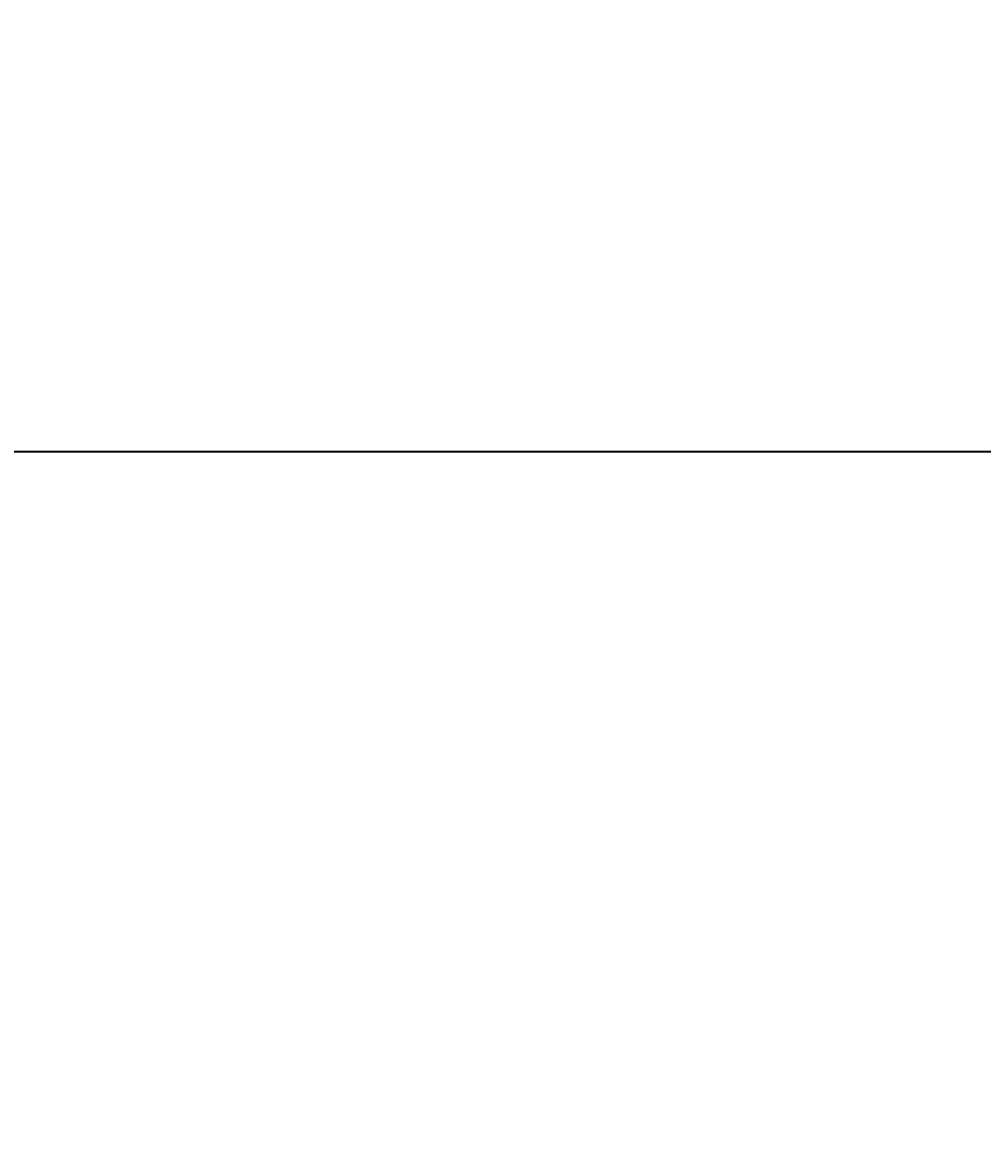
# Model space of a CAD drawing. Units: inches. Extents: x -26 to 776, y -22 to 650.
# Tile 28 of 62: x 94 to 192, y 420 to 535. Entities that reach past the tile are written whole.
import ezdxf

# ---------------------------------------------------------------- set-up
doc = ezdxf.new("R2010")
doc.units = ezdxf.units.IN
doc.header["$MEASUREMENT"] = 0
doc.layers.add('A-ANNO-DIMS', color=2, linetype='Continuous', lineweight=18)
doc.layers.add('A-WALL', color=7, linetype='Continuous', lineweight=35)
doc.styles.get("Standard").update_dxf_attribs({"font": 'arial.ttf'})
doc.dimstyles.get("Standard").update_dxf_attribs({"dimtxt": 0.5625, "dimasz": 0.18, "dimexe": 0.18, "dimexo": 0.0625, "dimgap": 0.09, "dimtad": 0, "dimtih": 1, "dimtoh": 1, "dimdec": 4, "dimzin": 0, "dimdsep": 46, "dimlunit": 4, "dimtxsty": 'Standard', "dimcen": 0.09, "dimadec": 0, "dimazin": 0, "dimtfac": 1, "dimtdec": 4, "dimtofl": 0, "dimtmove": 0, "dimatfit": 3, "dimfxl": 1, "dimtolj": 1, "dimtzin": 0, "dimarcsym": 0})

# ---------------------------------------------------------------- blocks, each defined once
blk = doc.blocks.new('*D14')
at = {"layer": 'A-ANNO-DIMS', "color": 0, "lineweight": -2, "transparency": 16777216}
for p, q in [((191.62, 613.27), (-25.48, 613.27)), ((-25.3, 613.09), (-25.3, 314.75)), ((-25.3, 15.66), (-25.3, 314)), ((11.04, 15.48), (-25.48, 15.48))]:
    blk.add_line(p, q, dxfattribs=at)
at = {"layer": 'A-ANNO-DIMS', "color": 0, "transparency": 16777216}
for points in [[(-25.33, 613.09), (-25.27, 613.09), (-25.3, 613.27)], [(-25.33, 15.66), (-25.27, 15.66), (-25.3, 15.48)]]:
    blk.add_solid(points, dxfattribs=at)
at = {"layer": 'Defpoints', "color": 0, "transparency": 16777216}
for p in [(-25.3, 613.27), (191.68, 613.27), (11.11, 15.48)]:
    blk.add_point(p, dxfattribs=at)
at = {"layer": 'A-ANNO-DIMS', "color": 0, "transparency": 16777216, "insert": (-25.3, 314.38), "char_height": 0.562, "attachment_point": 5}
blk.add_mtext('\\A1;597.8', dxfattribs=at)
blk = doc.blocks.new('*D15')
at = {"layer": 'A-ANNO-DIMS', "color": 0, "lineweight": -2, "transparency": 16777216}
for p, q in [((11.11, 491.49), (11.11, 649.86)), ((11.29, 649.68), (120.22, 649.68)), ((231.24, 649.68), (122.31, 649.68)), ((231.42, 491.49), (231.42, 649.86))]:
    blk.add_line(p, q, dxfattribs=at)
at = {"layer": 'A-ANNO-DIMS', "color": 0, "transparency": 16777216}
for points in [[(11.29, 649.71), (11.29, 649.65), (11.11, 649.68)], [(231.24, 649.71), (231.24, 649.65), (231.42, 649.68)]]:
    blk.add_solid(points, dxfattribs=at)
at = {"layer": 'Defpoints', "color": 0, "transparency": 16777216}
for p in [(231.42, 649.68), (11.11, 491.43), (231.42, 491.43)]:
    blk.add_point(p, dxfattribs=at)
at = {"layer": 'A-ANNO-DIMS', "color": 0, "transparency": 16777216, "insert": (121.27, 649.68), "char_height": 0.562, "attachment_point": 5}
blk.add_mtext('\\A1;220.3', dxfattribs=at)
blk = doc.blocks.new('*D17')
at = {"layer": 'A-ANNO-DIMS', "color": 0, "lineweight": -2, "transparency": 16777216}
for p, q in [((11.11, 491.49), (11.11, 649.86)), ((11.29, 649.68), (100.16, 649.68)), ((191.5, 649.68), (102.62, 649.68)), ((191.68, 613.33), (191.68, 649.86))]:
    blk.add_line(p, q, dxfattribs=at)
at = {"layer": 'A-ANNO-DIMS', "color": 0, "transparency": 16777216}
for points in [[(11.29, 649.71), (11.29, 649.65), (11.11, 649.68)], [(191.5, 649.71), (191.5, 649.65), (191.68, 649.68)]]:
    blk.add_solid(points, dxfattribs=at)
at = {"layer": 'Defpoints', "color": 0, "transparency": 16777216}
for p in [(191.68, 649.68), (191.68, 613.27), (11.11, 491.43)]:
    blk.add_point(p, dxfattribs=at)
at = {"layer": 'A-ANNO-DIMS', "color": 0, "transparency": 16777216, "insert": (101.39, 649.68), "char_height": 0.562, "attachment_point": 5}
blk.add_mtext('\\A1;180.57', dxfattribs=at)
blk = doc.blocks.new('*D19')
at = {"layer": 'A-ANNO-DIMS', "color": 0, "lineweight": -2, "transparency": 16777216}
for p, q in [((191.62, 613.27), (-25.48, 613.27)), ((-25.3, 613.09), (-25.3, 552.73)), ((-25.3, 491.61), (-25.3, 551.97)), ((191.62, 491.43), (-25.48, 491.43))]:
    blk.add_line(p, q, dxfattribs=at)
at = {"layer": 'A-ANNO-DIMS', "color": 0, "transparency": 16777216}
for points in [[(-25.33, 613.09), (-25.27, 613.09), (-25.3, 613.27)], [(-25.33, 491.61), (-25.27, 491.61), (-25.3, 491.43)]]:
    blk.add_solid(points, dxfattribs=at)
at = {"layer": 'Defpoints', "color": 0, "transparency": 16777216}
for p in [(-25.3, 613.27), (191.68, 613.27), (191.68, 491.43)]:
    blk.add_point(p, dxfattribs=at)
at = {"layer": 'A-ANNO-DIMS', "color": 0, "transparency": 16777216, "insert": (-25.3, 552.35), "char_height": 0.562, "attachment_point": 5}
blk.add_mtext('\\A1;121.84', dxfattribs=at)
blk = doc.blocks.new('*D22')
at = {"layer": 'A-ANNO-DIMS', "color": 0, "lineweight": -2, "transparency": 16777216}
for p, q in [((22.89, 15.33), (22.89, 649.86)), ((23.07, 649.68), (119.19, 649.68)), ((217.77, 649.68), (121.65, 649.68)), ((217.95, 15.54), (217.95, 649.86))]:
    blk.add_line(p, q, dxfattribs=at)
at = {"layer": 'A-ANNO-DIMS', "color": 0, "transparency": 16777216}
for points in [[(23.07, 649.71), (23.07, 649.65), (22.89, 649.68)], [(217.77, 649.71), (217.77, 649.65), (217.95, 649.68)]]:
    blk.add_solid(points, dxfattribs=at)
at = {"layer": 'Defpoints', "color": 0, "transparency": 16777216}
for p in [(217.95, 649.68), (22.89, 15.27), (217.95, 15.48)]:
    blk.add_point(p, dxfattribs=at)
at = {"layer": 'A-ANNO-DIMS', "color": 0, "transparency": 16777216, "insert": (120.42, 649.68), "char_height": 0.562, "attachment_point": 5}
blk.add_mtext('\\A1;195.06', dxfattribs=at)
blk = doc.blocks.new('*D35')
at = {"layer": 'A-ANNO-DIMS', "color": 0, "lineweight": -2, "transparency": 16777216}
for p, q in [((82.13, 420.34), (82.13, 649.86)), ((82.31, 649.68), (144.38, 649.68)), ((208.91, 649.68), (146.84, 649.68)), ((209.09, 420.34), (209.09, 649.86))]:
    blk.add_line(p, q, dxfattribs=at)
at = {"layer": 'A-ANNO-DIMS', "color": 0, "transparency": 16777216}
for points in [[(82.31, 649.71), (82.31, 649.65), (82.13, 649.68)], [(208.91, 649.71), (208.91, 649.65), (209.09, 649.68)]]:
    blk.add_solid(points, dxfattribs=at)
at = {"layer": 'Defpoints', "color": 0, "transparency": 16777216}
for p in [(209.09, 649.68), (82.13, 420.28), (209.09, 420.28)]:
    blk.add_point(p, dxfattribs=at)
at = {"layer": 'A-ANNO-DIMS', "color": 0, "transparency": 16777216, "insert": (145.61, 649.68), "char_height": 0.562, "attachment_point": 5}
blk.add_mtext('\\A1;126.96', dxfattribs=at)

msp = doc.modelspace()

# ---------------------------------------------------------------- linework, layer by layer
at = {"layer": 'A-WALL'}
msp.add_line((11.1074, 491.4269), (231.4249, 491.4269), dxfattribs=at)

# ---------------------------------------------------------------- dimensions: what is measured, and where the dimension line sits
at = {"layer": 'A-ANNO-DIMS'}
for base, p1, p2, override, picture, middle in [((231.4249, 649.6763), (11.1074, 491.4269), (231.4249, 491.4269), {"dimdec": 1, "dimlfac": 1, "dimrnd": 0, "dimzin": 0, "dimdsep": 46, "dimlunit": 2}, '*D15', (121.2661, 649.6763)), ((191.6782, 649.6763), (11.1074, 491.4269), (191.6782, 613.2713), {"dimdec": 2, "dimlfac": 1, "dimrnd": 0, "dimzin": 0, "dimdsep": 46, "dimlunit": 2}, '*D17', (101.3928, 649.6763)), ((217.9529, 649.6763), (22.8891, 15.2701), (217.9529, 15.4824), {"dimdec": 2, "dimlfac": 1, "dimrnd": 0, "dimzin": 0, "dimdsep": 46, "dimlunit": 2}, '*D22', (120.421, 649.6763)), ((209.091, 649.6763), (82.134, 420.2783), (209.091, 420.2783), {"dimdec": 2, "dimlfac": 1, "dimrnd": 0, "dimzin": 0, "dimdsep": 46, "dimlunit": 2}, '*D35', (145.6125, 649.6763))]:
    dim = msp.add_linear_dim(base=base, p1=p1, p2=p2, dimstyle='Standard', override=override, dxfattribs=at)
    dim.commit()
    dim.dimension.update_dxf_attribs({"geometry": picture, "text_midpoint": middle})
for p1, override, picture, middle in [((191.6782, 491.4269), {"dimdec": 2, "dimlfac": 1, "dimrnd": 0, "dimzin": 0, "dimdsep": 46, "dimlunit": 2}, '*D19', (-25.2976, 552.3491)), ((11.1074, 15.4824), {"dimdec": 1, "dimlfac": 1, "dimrnd": 0, "dimzin": 0, "dimdsep": 46, "dimlunit": 2}, '*D14', (-25.2976, 314.3769))]:
    dim = msp.add_linear_dim(base=(-25.2976, 613.2713), p1=p1, p2=(191.6782, 613.2713), angle=90, dimstyle='Standard', override=override, dxfattribs=at)
    dim.commit()
    dim.dimension.update_dxf_attribs({"geometry": picture, "text_midpoint": middle})

doc.saveas('drawing.dxf')
